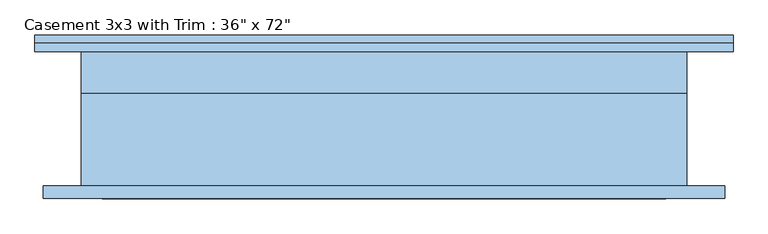
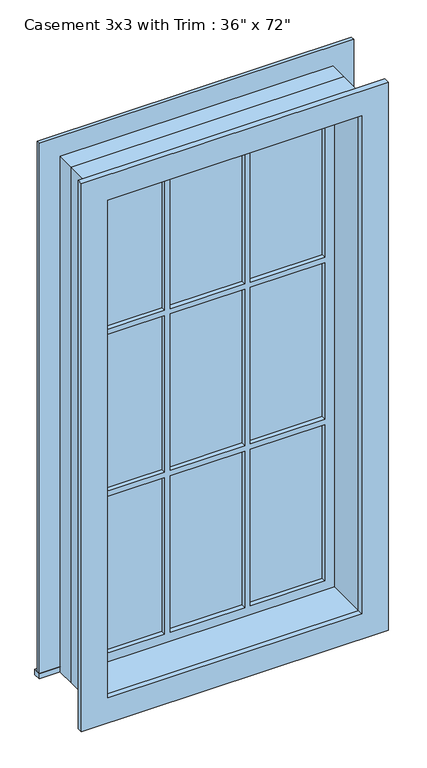
"""IFC4 building model written with IfcOpenShell, lengths in millimetres: window geometry."""

from ifc_helpers import new_model, si_unit, frame, origin, place, context, project, spatial, polyline, outline, extrude, source, transform, mapped, element, save


def window_8b323df3(model_context):
    return source(origin(), model_context, "Body", "SweptSolid", [
        extrude(outline(polyline([(-527.05, 127.0), (527.05, 127.0), (527.05, 101.6), (-527.05, 101.6), (-527.05, 127.0)])), frame((0.0, 0.0, 304.8), z_axis=(0.0, 0.0, 1.0), x_axis=(1.0, 0.0, 0.0)), (0.0, 0.0, 1.0), 19.05),
        extrude(outline(polyline([(2114.55, -438.15), (2114.55, 438.15), (323.85, 438.15), (323.85, 527.05), (2203.45, 527.05), (2203.45, -527.05), (323.85, -527.05), (323.85, -438.15), (2114.55, -438.15)])), frame((0.0, 101.6, 0.0), z_axis=(0.0, 1.0, 0.0), x_axis=(0.0, 0.0, 1.0)), (0.0, 0.0, 1.0), 12.7),
        extrude(outline(polyline([(143.9333333, 66.675), (393.7, 66.675), (393.7, 53.975), (143.9333333, 53.975), (143.9333333, 66.675)])), frame((0.0, 0.0, 1515.5333333), z_axis=(0.0, 0.0, 1.0), x_axis=(1.0, 0.0, 0.0)), (0.0, 0.0, 1.0), 554.5666667),
        extrude(outline(polyline([(-124.8833333, 66.675), (124.8833333, 66.675), (124.8833333, 53.975), (-124.8833333, 53.975), (-124.8833333, 66.675)])), frame((0.0, 0.0, 1515.5333333), z_axis=(0.0, 0.0, 1.0), x_axis=(1.0, 0.0, 0.0)), (0.0, 0.0, 1.0), 554.5666667),
        extrude(outline(polyline([(-393.7, 66.675), (-143.9333333, 66.675), (-143.9333333, 53.975), (-393.7, 53.975), (-393.7, 66.675)])), frame((0.0, 0.0, 1515.5333333), z_axis=(0.0, 0.0, 1.0), x_axis=(1.0, 0.0, 0.0)), (0.0, 0.0, 1.0), 554.5666667),
        extrude(outline(polyline([(-393.7, 66.675), (-143.9333333, 66.675), (-143.9333333, 53.975), (-393.7, 53.975), (-393.7, 66.675)])), frame((0.0, 0.0, 941.9166667), z_axis=(0.0, 0.0, 1.0), x_axis=(1.0, 0.0, 0.0)), (0.0, 0.0, 1.0), 554.5666667),
        extrude(outline(polyline([(-124.8833333, 66.675), (124.8833333, 66.675), (124.8833333, 53.975), (-124.8833333, 53.975), (-124.8833333, 66.675)])), frame((0.0, 0.0, 941.9166667), z_axis=(0.0, 0.0, 1.0), x_axis=(1.0, 0.0, 0.0)), (0.0, 0.0, 1.0), 554.5666667),
        extrude(outline(polyline([(143.9333333, 66.675), (393.7, 66.675), (393.7, 53.975), (143.9333333, 53.975), (143.9333333, 66.675)])), frame((0.0, 0.0, 941.9166667), z_axis=(0.0, 0.0, 1.0), x_axis=(1.0, 0.0, 0.0)), (0.0, 0.0, 1.0), 554.5666667),
        extrude(outline(polyline([(143.9333333, 66.675), (393.7, 66.675), (393.7, 53.975), (143.9333333, 53.975), (143.9333333, 66.675)])), frame((0.0, 0.0, 368.3), z_axis=(0.0, 0.0, 1.0), x_axis=(1.0, 0.0, 0.0)), (0.0, 0.0, 1.0), 554.5666667),
        extrude(outline(polyline([(-124.8833333, 66.675), (124.8833333, 66.675), (124.8833333, 53.975), (-124.8833333, 53.975), (-124.8833333, 66.675)])), frame((0.0, 0.0, 368.3), z_axis=(0.0, 0.0, 1.0), x_axis=(1.0, 0.0, 0.0)), (0.0, 0.0, 1.0), 554.5666667),
        extrude(outline(polyline([(-393.7, 66.675), (-143.9333333, 66.675), (-143.9333333, 53.975), (-393.7, 53.975), (-393.7, 66.675)])), frame((0.0, 0.0, 368.3), z_axis=(0.0, 0.0, 1.0), x_axis=(1.0, 0.0, 0.0)), (0.0, 0.0, 1.0), 554.5666667),
        extrude(outline(polyline([(2190.75, 514.35), (2190.75, -514.35), (247.65, -514.35), (247.65, 514.35), (2190.75, 514.35)]), holes=[polyline([(2101.85, 425.45), (336.55, 425.45), (336.55, -425.45), (2101.85, -425.45), (2101.85, 425.45)])]), frame((0.0, -120.65, 0.0), z_axis=(0.0, 1.0, 0.0), x_axis=(0.0, 0.0, 1.0)), (0.0, 0.0, 1.0), 19.05),
        extrude(outline(polyline([(2114.55, -438.15), (323.85, -438.15), (323.85, 438.15), (2114.55, 438.15), (2114.55, -438.15)]), holes=[polyline([(2070.1, -143.9333333), (1515.5333333, -143.9333333), (1515.5333333, -393.7), (2070.1, -393.7), (2070.1, -143.9333333)]), polyline([(1496.4833333, -143.9333333), (941.9166667, -143.9333333), (941.9166667, -393.7), (1496.4833333, -393.7), (1496.4833333, -143.9333333)]), polyline([(922.8666667, -143.9333333), (368.3, -143.9333333), (368.3, -393.7), (922.8666667, -393.7), (922.8666667, -143.9333333)]), polyline([(2070.1, 124.8833333), (1515.5333333, 124.8833333), (1515.5333333, -124.8833333), (2070.1, -124.8833333), (2070.1, 124.8833333)]), polyline([(1496.4833333, 124.8833333), (941.9166667, 124.8833333), (941.9166667, -124.8833333), (1496.4833333, -124.8833333), (1496.4833333, 124.8833333)]), polyline([(922.8666667, 124.8833333), (368.3, 124.8833333), (368.3, -124.8833333), (922.8666667, -124.8833333), (922.8666667, 124.8833333)]), polyline([(2070.1, 393.7), (1515.5333333, 393.7), (1515.5333333, 143.9333333), (2070.1, 143.9333333), (2070.1, 393.7)]), polyline([(1496.4833333, 393.7), (941.9166667, 393.7), (941.9166667, 143.9333333), (1496.4833333, 143.9333333), (1496.4833333, 393.7)]), polyline([(922.8666667, 393.7), (368.3, 393.7), (368.3, 143.9333333), (922.8666667, 143.9333333), (922.8666667, 393.7)])]), frame((0.0, 38.1, 0.0), z_axis=(0.0, 1.0, 0.0), x_axis=(0.0, 0.0, 1.0)), (0.0, 0.0, 1.0), 44.45),
        extrude(outline(polyline([(2133.6, -457.2), (304.8, -457.2), (304.8, 457.2), (2133.6, 457.2), (2133.6, -457.2)]), holes=[polyline([(2101.85, -425.45), (2101.85, 425.45), (336.55, 425.45), (336.55, -425.45), (2101.85, -425.45)])]), frame((0.0, -101.6, 0.0), z_axis=(0.0, 1.0, 0.0), x_axis=(0.0, 0.0, 1.0)), (0.0, 0.0, 1.0), 139.7),
        extrude(outline(polyline([(2133.6, 457.2), (2133.6, -457.2), (304.8, -457.2), (304.8, 457.2), (2133.6, 457.2)]), holes=[polyline([(2114.55, 438.15), (323.85, 438.15), (323.85, -438.15), (2114.55, -438.15), (2114.55, 438.15)])]), frame((0.0, 38.1, 0.0), z_axis=(0.0, 1.0, 0.0), x_axis=(0.0, 0.0, 1.0)), (0.0, 0.0, 1.0), 63.5),
    ])


if __name__ == "__main__":
    model = new_model("IFC4")
    model_context = context("Model", 3, world=origin())
    ifc_project = project(units=[si_unit("LENGTHUNIT", "METRE", prefix="MILLI")], contexts=[model_context])
    site = spatial("IfcSite", under=ifc_project)
    building = spatial("IfcBuilding", under=site)
    placement = place(None, origin())
    window_shape = window_8b323df3(model_context)
    element("IfcWindow", 1, ObjectType="Casement 3x3 with Trim : 36\" x 72\"", at=placement, inside=building, context=model_context, shape_type="MappedRepresentation", body=[
        mapped(window_shape, transform((0.0, 0.0, 0.0), x_axis=(1.0, 0.0, 0.0), y_axis=(0.0, 1.0, 0.0), z_axis=(0.0, 0.0, 1.0))),
    ])
    save(model, "model.ifc")

# Revit data of these elements
# Type "Casement 3x3 with Trim : 36\" x 72\""
#   Type Mark = "12"
#   Construction Type Id = "GSP4R"
#   Assembly Code = "B2020100"
#   Analytic Construction = "1/8 in Pilkington single glazing"
#   Visual Light Transmittance = 0.9
#   Solar Heat Gain Coefficient = 0.78
#   Heat Transfer Coefficient (U) = 0.6496 BTU/(h·ft²·°F)
#   Height = 6' - 0"
#   Default Sill Height = 1' - 0"
#   Trim Projection - Ext. = 0' - 0 1/2"
#   Trim Projection - Int. = 0' - 0 3/4"
#   Trim Width - Exterior = 0' - 3 1/2"
#   Trim Width - Interior = 0' - 3 1/2"
#   Width = 3' - 0"
#   Window Inset = 0' - 0 3/4"
#   Define Thermal Properties by = 1
#   Glass Pane Material = Glass
#   Sash Material = Sash
#   Trim Exterior Material = Trim
#   Trim Interior Material = Trim
#   Wall Closure = (empty or 0)
# Element 1 (IfcWindow, "Casement 3x3 with Trim : 36\" x 72\"")
#   Materials on its faces: "Sash", "Glass", "Trim"
# Materials
#   "Glass": class "Glass", colour RGB 0 128 192, transparency 0.75, Description = "Soda Lime Glass", Cost = 0
#   "Sash": class "Wood", colour RGB 224 178 126, transparency 0
#   "Trim": class "Wood", colour RGB 224 178 126, transparency 0
